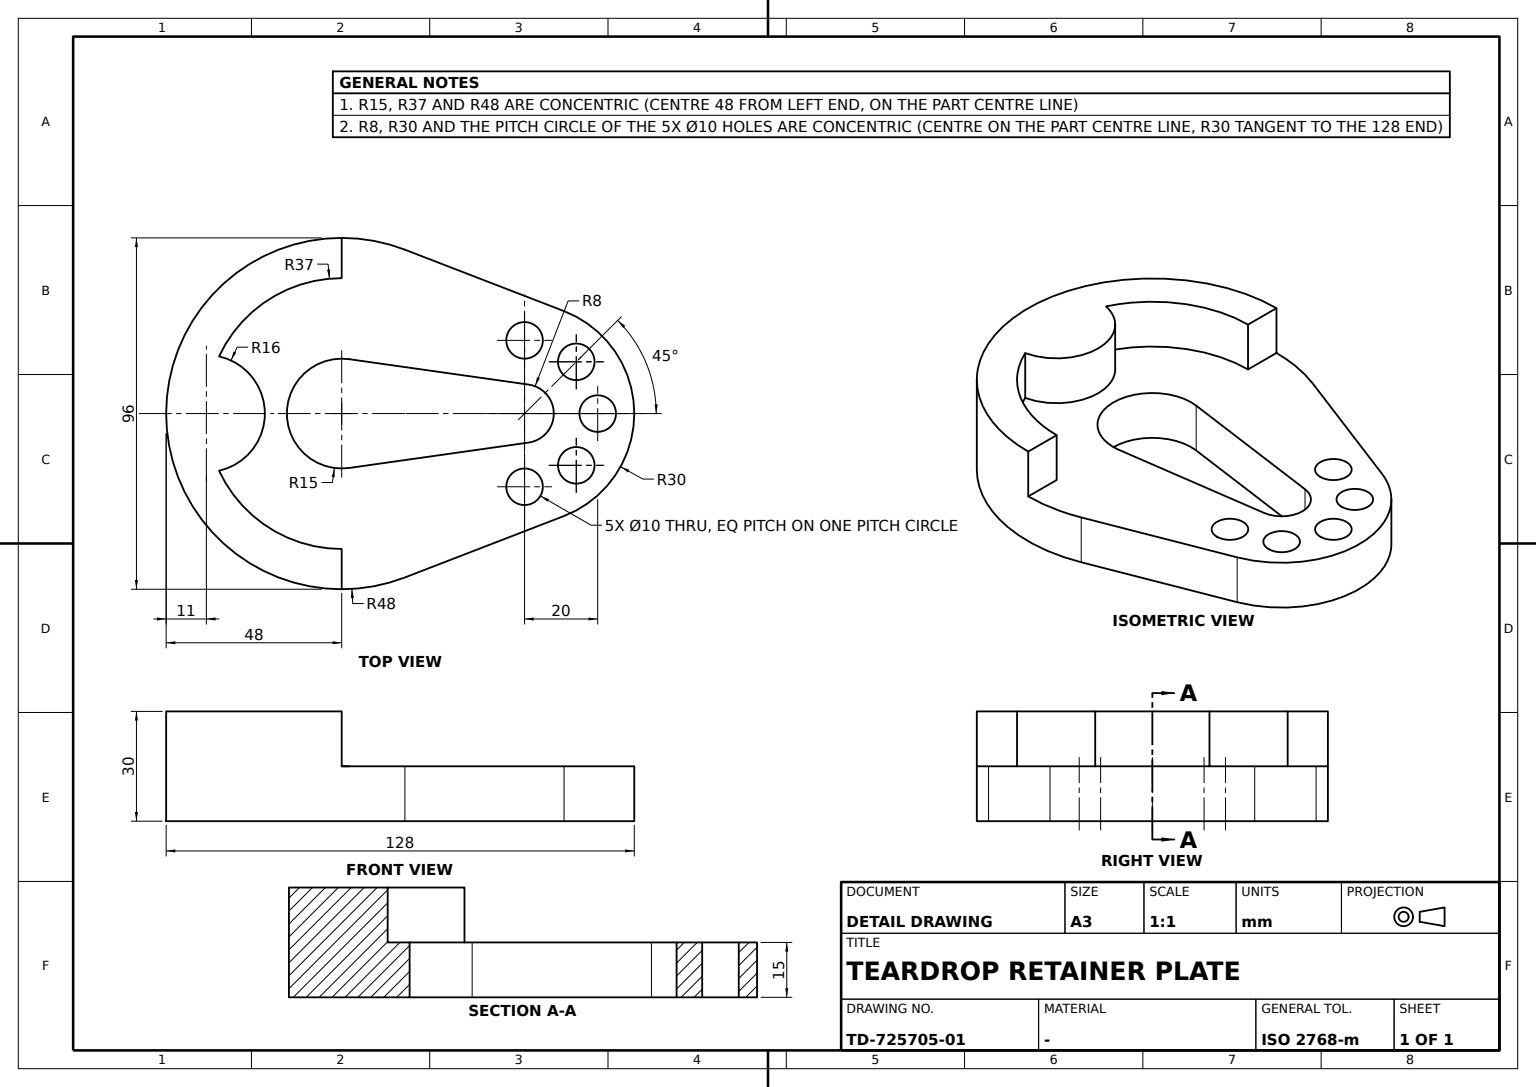
CATIA V5 part; units mm, degrees
sketch "Sketch1" plane through (0, 0, 0) normal (0, 0, 1) x (1, 0, 0)
  line L0 (0, 0) -> (0, 50) construction
  point P0 (0, 50)
  line L1 (-44.7817, 17.28) -> (-27.9886, 60.8)
  line L2 (27.9886, 60.8) -> (44.7817, 17.28)
  arc A0 (-27.9886, 60.8) -> (27.9886, 60.8) centre (0, 50) cw
  arc A1 (44.7817, 17.28) -> (-44.7817, 17.28) centre (0, 0) cw
  line L3 (0, 0) -> (0, 50) construction
  line L4 (-14.8523, 2.1) -> (-7.9212, 51.12)
  line L5 (7.9212, 51.12) -> (14.8523, 2.1)
  arc A2 (-7.9212, 51.12) -> (7.9212, 51.12) centre (0, 50) cw
  arc A3 (14.8523, 2.1) -> (-14.8523, 2.1) centre (0, 0) cw
  circle A4 centre (0, 50) radius 20 construction
  point P1 (0, 50)
  line L6 (0, 50) -> (74.8892, 50) construction
  line L7 (0, 50) -> (-67.5194, 50) construction
  circle A5 centre (20, 50) radius 5
  point P2 (20, 50)
  circle A6 centre (-20, 50) radius 5
  point P3 (-20, 50)
  point P4 (14.1421, 64.1421)
  circle A7 centre (14.1421, 64.1421) radius 5
  point P5 (0, 70)
  circle A8 centre (0, 70) radius 5
  point P6 (-14.1421, 64.1421)
  circle A9 centre (-14.1421, 64.1421) radius 5
  line L8 (0, 50) -> (0, 114.3359) construction
  line L9 (0, 50) -> (25.8854, 75.8854) construction
  line L10 (0, 50) -> (-24.4101, 74.4101) construction
  point P7 (0, 50)
  dimension "radius A1" = 48
  dimension "radius A0" = 30
  dimension "radius A3" = 15
  dimension "radius A2" = 8
  dimension "radius A4" = 20
  dimension "radius A5" = 5
  dimension "radius A6" = 5
  dimension "radius A7" = 5
  dimension "radius A8" = 5
  dimension "radius A9" = 5
  dimension "angle L9 L8" = 45
  dimension "angle L10 L8" = 45
  dimension "length L3" = 50
  constraint vertical L0 y-axis
  constraint vertical L3 y-axis
  constraint vertical L8 y-axis
  constraint tangency A0 L1
  constraint tangency A1 L1
  constraint tangency A0 L2
  constraint tangency A1 L2
  constraint tangency A2 L4
  constraint tangency A3 L4
  constraint tangency A2 L5
  constraint tangency A3 L5
  constraint coincidence P1 y-axis
  constraint coincidence P2 L6
  constraint coincidence P2 A4
  constraint coincidence P0 L6
  constraint coincidence P3 L7
  constraint coincidence P3 A4
  constraint coincidence P4 A4
  constraint coincidence P5 A4
  constraint coincidence P6 A4
  constraint coincidence P5 L8
  constraint coincidence L9 P4
  constraint coincidence P7 L9
  constraint coincidence P7 L6
  constraint coincidence L10 P6
  constraint horizontal L6 x-axis
  constraint horizontal L7 x-axis
extrude "Pad1" add sketch "Sketch1" against normal blind 15
sketch "Sketch2" plane through (0, 0, 0) normal (0, 0, 1) x (1, 0, 0)
  arc A0 (-48, 0) -> (48, 0) centre (0, 0) ccw
  arc A1 (-46.7396, 10.9273) -> (46.7396, 10.9273) centre (0, 0) ccw construction
  arc A2 (-37, 0) -> (-15.6215, -33.5405) centre (0, 0) ccw
  arc A3 (15.6215, -33.5405) -> (-15.6215, -33.5405) centre (0, -37) ccw
  point P0 (0, -37)
  line L0 (48, 0) -> (37, 0)
  point P1 (-37, 0)
  line L1 (-37, 0) -> (-48, 0)
  arc A4 (15.6215, -33.5405) -> (37, 0) centre (0, 0) ccw
  dimension "radius A2" = 37
  dimension "radius A3" = 16
  dimension "distance L0 x axis" = 0
  constraint coincidence A0 A1
  constraint coincidence P0 A2
  constraint coincidence P0 y-axis
  constraint coincidence L0 P1
  constraint coincidence L0 L1
  constraint coincidence A2 A4
  constraint horizontal L0 x-axis
  constraint horizontal L1 x-axis
extrude "Pad2" add sketch "Sketch2" along normal blind 15
